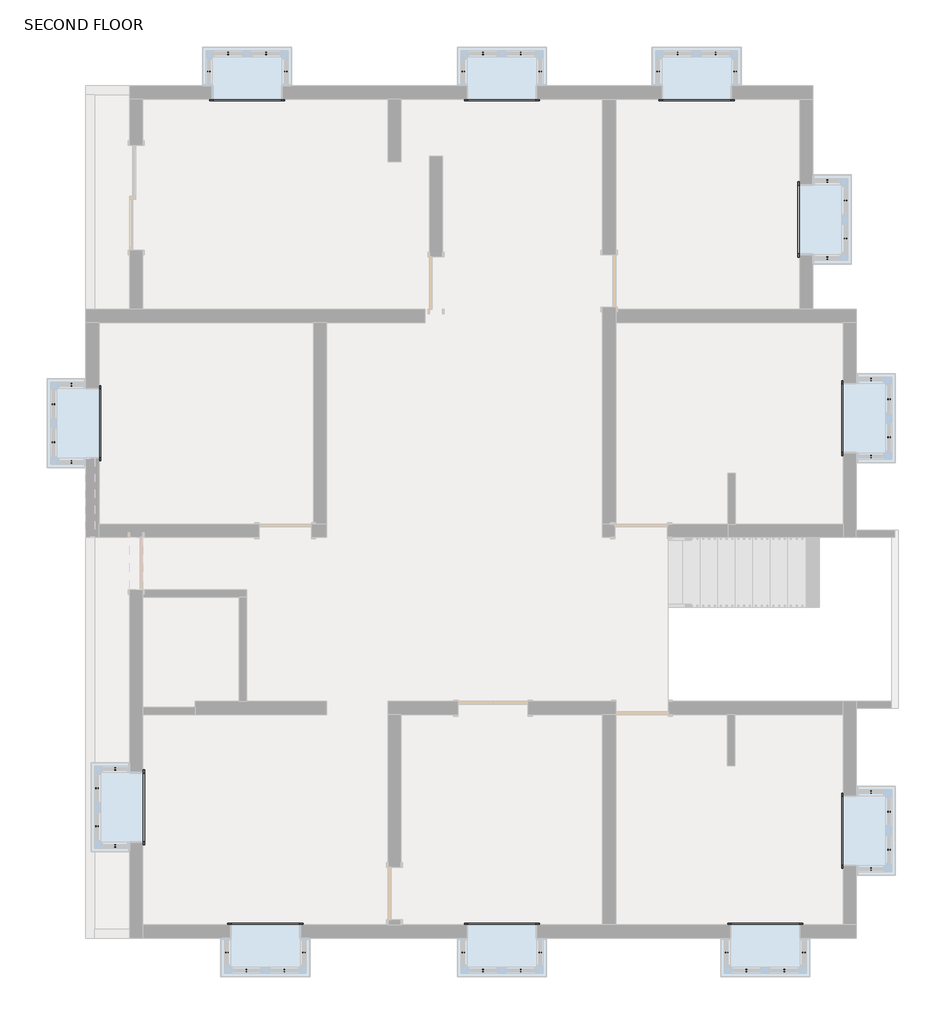
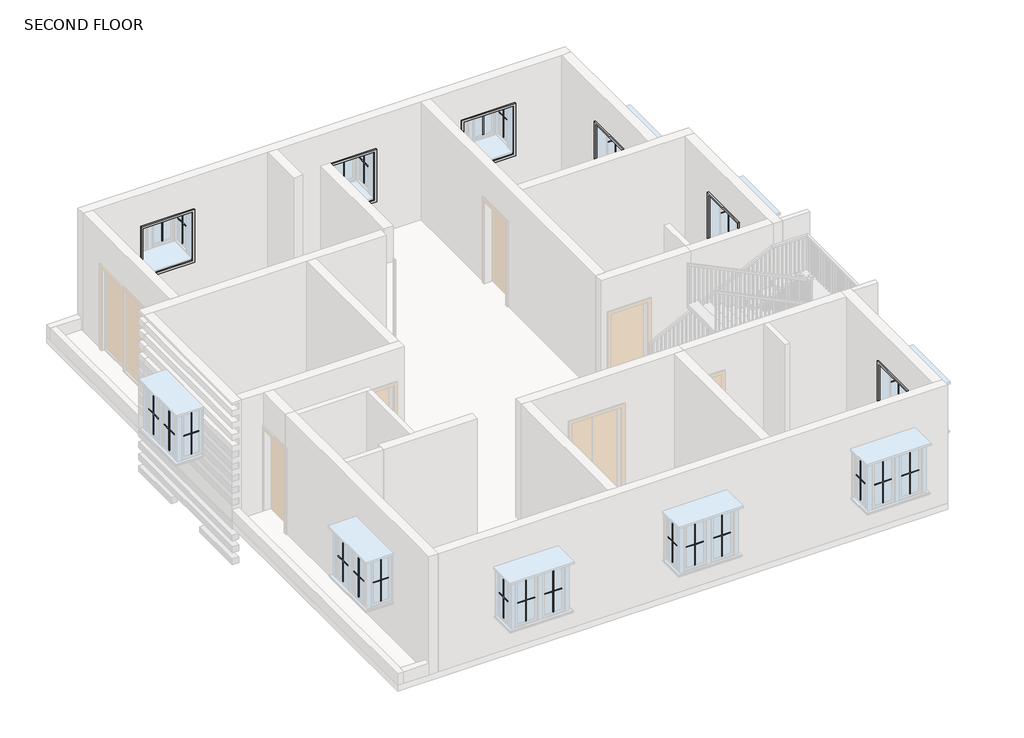
# One storey, part 6 of 6: 55 proxies.
"""IFC4 building model written with IfcOpenShell, lengths in millimetres."""

from ifc_helpers import new_model, si_unit, origin, place, context, project, spatial, transform, mapped, element, save
from components import muntin_pattern_2x2_muntin_pattern_2x2_4aee108e, muntin_pattern_2x2_muntin_pattern_2x2_f03ab90d, muntin_pattern_2x2_muntin_pattern_2x2_eb08c668, trim_window_interior_flat_picture_frame_ace0ae79

model = new_model("IFC4")

# Units and contexts
model_context = context("Model", 3, world=origin())
ifc_project = project(units=[si_unit("LENGTHUNIT", "METRE", prefix="MILLI")], contexts=[model_context])

# Site, building, storey
site = spatial("IfcSite", under=ifc_project)
building = spatial("IfcBuilding", under=site)
storey = spatial("IfcBuildingStorey", under=building, Name="SECOND FLOOR", Elevation=6400.8)

# Proxies
placement = place(None, origin())
muntin_pattern_2x2_muntin_pattern_2x2_shape = muntin_pattern_2x2_muntin_pattern_2x2_4aee108e(model_context)
element("IfcBuildingElementProxy", 1, Name="Muntin Pattern_2x2 : Muntin Pattern_2x2", ObjectType="Muntin Pattern_2x2 : Muntin Pattern_2x2", at=placement, inside=storey, context=model_context, shape_type="MappedRepresentation", body=[
    mapped(muntin_pattern_2x2_muntin_pattern_2x2_shape, transform((6209.1834916, 6075.433346, 7435.85), x_axis=(0.0, -1.0, 0.0), y_axis=(1.0, 0.0, 0.0), z_axis=(0.0, 0.0, 1.0))),
])
element("IfcBuildingElementProxy", 2, Name="Muntin Pattern_2x2 : Muntin Pattern_2x2", ObjectType="Muntin Pattern_2x2 : Muntin Pattern_2x2", at=placement, inside=storey, context=model_context, shape_type="MappedRepresentation", body=[
    mapped(muntin_pattern_2x2_muntin_pattern_2x2_shape, transform((-99.5415084, 8637.658346, 7435.85), x_axis=(1.0, 0.0, 0.0), y_axis=(0.0, 1.0, 0.0), z_axis=(0.0, 0.0, 1.0))),
])
element("IfcBuildingElementProxy", 3, Name="Muntin Pattern_2x2 : Muntin Pattern_2x2", ObjectType="Muntin Pattern_2x2 : Muntin Pattern_2x2", at=placement, inside=storey, context=model_context, shape_type="MappedRepresentation", body=[
    mapped(muntin_pattern_2x2_muntin_pattern_2x2_shape, transform((3291.3584916, 8637.658346, 7435.85), x_axis=(1.0, 0.0, 0.0), y_axis=(0.0, 1.0, 0.0), z_axis=(0.0, 0.0, 1.0))),
])
element("IfcBuildingElementProxy", 4, Name="Muntin Pattern_2x2 : Muntin Pattern_2x2", ObjectType="Muntin Pattern_2x2 : Muntin Pattern_2x2", at=placement, inside=storey, context=model_context, shape_type="MappedRepresentation", body=[
    mapped(muntin_pattern_2x2_muntin_pattern_2x2_shape, transform((-4531.8415084, 8637.658346, 7435.85), x_axis=(1.0, 0.0, 0.0), y_axis=(0.0, 1.0, 0.0), z_axis=(0.0, 0.0, 1.0))),
])
element("IfcBuildingElementProxy", 5, Name="Muntin Pattern_2x2 : Muntin Pattern_2x2", ObjectType="Muntin Pattern_2x2 : Muntin Pattern_2x2", at=placement, inside=storey, context=model_context, shape_type="MappedRepresentation", body=[
    mapped(muntin_pattern_2x2_muntin_pattern_2x2_shape, transform((-7576.6665084, 1871.733346, 7435.85), x_axis=(0.0, 1.0, 0.0), y_axis=(-1.0, 0.0, 0.0), z_axis=(0.0, 0.0, 1.0))),
])
element("IfcBuildingElementProxy", 6, Name="Muntin Pattern_2x2 : Muntin Pattern_2x2", ObjectType="Muntin Pattern_2x2 : Muntin Pattern_2x2", at=placement, inside=storey, context=model_context, shape_type="MappedRepresentation", body=[
    mapped(muntin_pattern_2x2_muntin_pattern_2x2_shape, transform((6971.1834916, 2621.033346, 7435.85), x_axis=(0.0, -1.0, 0.0), y_axis=(1.0, 0.0, 0.0), z_axis=(0.0, 0.0, 1.0))),
])
element("IfcBuildingElementProxy", 7, Name="Muntin Pattern_2x2 : Muntin Pattern_2x2", ObjectType="Muntin Pattern_2x2 : Muntin Pattern_2x2", at=placement, inside=storey, context=model_context, shape_type="MappedRepresentation", body=[
    mapped(muntin_pattern_2x2_muntin_pattern_2x2_shape, transform((-3553.9415084, -7319.891654, 7435.85), x_axis=(-1.0, 0.0, 0.0), y_axis=(0.0, -1.0, 0.0), z_axis=(0.0, 0.0, 1.0))),
])
element("IfcBuildingElementProxy", 8, Name="Muntin Pattern_2x2 : Muntin Pattern_2x2", ObjectType="Muntin Pattern_2x2 : Muntin Pattern_2x2", at=placement, inside=storey, context=model_context, shape_type="MappedRepresentation", body=[
    mapped(muntin_pattern_2x2_muntin_pattern_2x2_shape, transform((5145.5584916, -7319.891654, 7435.85), x_axis=(-1.0, 0.0, 0.0), y_axis=(0.0, -1.0, 0.0), z_axis=(0.0, 0.0, 1.0))),
])
element("IfcBuildingElementProxy", 9, Name="Muntin Pattern_2x2 : Muntin Pattern_2x2", ObjectType="Muntin Pattern_2x2 : Muntin Pattern_2x2", at=placement, inside=storey, context=model_context, shape_type="MappedRepresentation", body=[
    mapped(muntin_pattern_2x2_muntin_pattern_2x2_shape, transform((560.8584916, -7319.891654, 7435.85), x_axis=(-1.0, 0.0, 0.0), y_axis=(0.0, -1.0, 0.0), z_axis=(0.0, 0.0, 1.0))),
])
element("IfcBuildingElementProxy", 10, Name="Muntin Pattern_2x2 : Muntin Pattern_2x2", ObjectType="Muntin Pattern_2x2 : Muntin Pattern_2x2", at=placement, inside=storey, context=model_context, shape_type="MappedRepresentation", body=[
    mapped(muntin_pattern_2x2_muntin_pattern_2x2_shape, transform((-6814.6665084, -4808.466654, 7435.85), x_axis=(0.0, 1.0, 0.0), y_axis=(-1.0, 0.0, 0.0), z_axis=(0.0, 0.0, 1.0))),
])
element("IfcBuildingElementProxy", 11, Name="Muntin Pattern_2x2 : Muntin Pattern_2x2", ObjectType="Muntin Pattern_2x2 : Muntin Pattern_2x2", at=placement, inside=storey, context=model_context, shape_type="MappedRepresentation", body=[
    mapped(muntin_pattern_2x2_muntin_pattern_2x2_shape, transform((6971.1834916, -4554.466654, 7435.85), x_axis=(0.0, -1.0, 0.0), y_axis=(1.0, 0.0, 0.0), z_axis=(0.0, 0.0, 1.0))),
])
muntin_pattern_2x2_muntin_pattern_2x2_2_shape = muntin_pattern_2x2_muntin_pattern_2x2_f03ab90d(model_context)
element("IfcBuildingElementProxy", 12, Name="Muntin Pattern_2x2 : Muntin Pattern_2x2", ObjectType="Muntin Pattern_2x2 : Muntin Pattern_2x2", at=placement, inside=storey, context=model_context, shape_type="MappedRepresentation", body=[
    mapped(muntin_pattern_2x2_muntin_pattern_2x2_2_shape, transform((5894.8584916, 6415.158346, 7435.85), x_axis=(-1.0, 0.0, 0.0), y_axis=(0.0, -1.0, 0.0), z_axis=(0.0, 0.0, 1.0))),
])
element("IfcBuildingElementProxy", 13, Name="Muntin Pattern_2x2 : Muntin Pattern_2x2", ObjectType="Muntin Pattern_2x2 : Muntin Pattern_2x2", at=placement, inside=storey, context=model_context, shape_type="MappedRepresentation", body=[
    mapped(muntin_pattern_2x2_muntin_pattern_2x2_2_shape, transform((5894.8584916, 5075.308346, 7435.85), x_axis=(1.0, 0.0, 0.0), y_axis=(0.0, 1.0, 0.0), z_axis=(0.0, 0.0, 1.0))),
])
element("IfcBuildingElementProxy", 14, Name="Muntin Pattern_2x2 : Muntin Pattern_2x2", ObjectType="Muntin Pattern_2x2 : Muntin Pattern_2x2", at=placement, inside=storey, context=model_context, shape_type="MappedRepresentation", body=[
    mapped(muntin_pattern_2x2_muntin_pattern_2x2_2_shape, transform((-439.2665084, 8323.333346, 7435.85), x_axis=(0.0, -1.0, 0.0), y_axis=(1.0, 0.0, 0.0), z_axis=(0.0, 0.0, 1.0))),
])
element("IfcBuildingElementProxy", 15, Name="Muntin Pattern_2x2 : Muntin Pattern_2x2", ObjectType="Muntin Pattern_2x2 : Muntin Pattern_2x2", at=placement, inside=storey, context=model_context, shape_type="MappedRepresentation", body=[
    mapped(muntin_pattern_2x2_muntin_pattern_2x2_2_shape, transform((900.5834916, 8323.333346, 7435.85), x_axis=(0.0, 1.0, 0.0), y_axis=(-1.0, 0.0, 0.0), z_axis=(0.0, 0.0, 1.0))),
])
element("IfcBuildingElementProxy", 16, Name="Muntin Pattern_2x2 : Muntin Pattern_2x2", ObjectType="Muntin Pattern_2x2 : Muntin Pattern_2x2", at=placement, inside=storey, context=model_context, shape_type="MappedRepresentation", body=[
    mapped(muntin_pattern_2x2_muntin_pattern_2x2_2_shape, transform((2951.6334916, 8323.333346, 7435.85), x_axis=(0.0, -1.0, 0.0), y_axis=(1.0, 0.0, 0.0), z_axis=(0.0, 0.0, 1.0))),
])
element("IfcBuildingElementProxy", 17, Name="Muntin Pattern_2x2 : Muntin Pattern_2x2", ObjectType="Muntin Pattern_2x2 : Muntin Pattern_2x2", at=placement, inside=storey, context=model_context, shape_type="MappedRepresentation", body=[
    mapped(muntin_pattern_2x2_muntin_pattern_2x2_2_shape, transform((4291.4834916, 8323.333346, 7435.85), x_axis=(0.0, 1.0, 0.0), y_axis=(-1.0, 0.0, 0.0), z_axis=(0.0, 0.0, 1.0))),
])
element("IfcBuildingElementProxy", 18, Name="Muntin Pattern_2x2 : Muntin Pattern_2x2", ObjectType="Muntin Pattern_2x2 : Muntin Pattern_2x2", at=placement, inside=storey, context=model_context, shape_type="MappedRepresentation", body=[
    mapped(muntin_pattern_2x2_muntin_pattern_2x2_2_shape, transform((-4871.5665084, 8323.333346, 7435.85), x_axis=(0.0, -1.0, 0.0), y_axis=(1.0, 0.0, 0.0), z_axis=(0.0, 0.0, 1.0))),
])
element("IfcBuildingElementProxy", 19, Name="Muntin Pattern_2x2 : Muntin Pattern_2x2", ObjectType="Muntin Pattern_2x2 : Muntin Pattern_2x2", at=placement, inside=storey, context=model_context, shape_type="MappedRepresentation", body=[
    mapped(muntin_pattern_2x2_muntin_pattern_2x2_2_shape, transform((-3531.7165084, 8323.333346, 7435.85), x_axis=(0.0, 1.0, 0.0), y_axis=(-1.0, 0.0, 0.0), z_axis=(0.0, 0.0, 1.0))),
])
element("IfcBuildingElementProxy", 20, Name="Muntin Pattern_2x2 : Muntin Pattern_2x2", ObjectType="Muntin Pattern_2x2 : Muntin Pattern_2x2", at=placement, inside=storey, context=model_context, shape_type="MappedRepresentation", body=[
    mapped(muntin_pattern_2x2_muntin_pattern_2x2_2_shape, transform((-7262.3415084, 1532.008346, 7435.85), x_axis=(1.0, 0.0, 0.0), y_axis=(0.0, 1.0, 0.0), z_axis=(0.0, 0.0, 1.0))),
])
element("IfcBuildingElementProxy", 21, Name="Muntin Pattern_2x2 : Muntin Pattern_2x2", ObjectType="Muntin Pattern_2x2 : Muntin Pattern_2x2", at=placement, inside=storey, context=model_context, shape_type="MappedRepresentation", body=[
    mapped(muntin_pattern_2x2_muntin_pattern_2x2_2_shape, transform((-7262.3415084, 2871.858346, 7435.85), x_axis=(-1.0, 0.0, 0.0), y_axis=(0.0, -1.0, 0.0), z_axis=(0.0, 0.0, 1.0))),
])
element("IfcBuildingElementProxy", 22, Name="Muntin Pattern_2x2 : Muntin Pattern_2x2", ObjectType="Muntin Pattern_2x2 : Muntin Pattern_2x2", at=placement, inside=storey, context=model_context, shape_type="MappedRepresentation", body=[
    mapped(muntin_pattern_2x2_muntin_pattern_2x2_2_shape, transform((6656.8584916, 2960.758346, 7435.85), x_axis=(-1.0, 0.0, 0.0), y_axis=(0.0, -1.0, 0.0), z_axis=(0.0, 0.0, 1.0))),
])
element("IfcBuildingElementProxy", 23, Name="Muntin Pattern_2x2 : Muntin Pattern_2x2", ObjectType="Muntin Pattern_2x2 : Muntin Pattern_2x2", at=placement, inside=storey, context=model_context, shape_type="MappedRepresentation", body=[
    mapped(muntin_pattern_2x2_muntin_pattern_2x2_2_shape, transform((6656.8584916, 1620.908346, 7435.85), x_axis=(1.0, 0.0, 0.0), y_axis=(0.0, 1.0, 0.0), z_axis=(0.0, 0.0, 1.0))),
])
element("IfcBuildingElementProxy", 24, Name="Muntin Pattern_2x2 : Muntin Pattern_2x2", ObjectType="Muntin Pattern_2x2 : Muntin Pattern_2x2", at=placement, inside=storey, context=model_context, shape_type="MappedRepresentation", body=[
    mapped(muntin_pattern_2x2_muntin_pattern_2x2_2_shape, transform((-3214.2165084, -7005.566654, 7435.85), x_axis=(0.0, 1.0, 0.0), y_axis=(-1.0, 0.0, 0.0), z_axis=(0.0, 0.0, 1.0))),
])
element("IfcBuildingElementProxy", 25, Name="Muntin Pattern_2x2 : Muntin Pattern_2x2", ObjectType="Muntin Pattern_2x2 : Muntin Pattern_2x2", at=placement, inside=storey, context=model_context, shape_type="MappedRepresentation", body=[
    mapped(muntin_pattern_2x2_muntin_pattern_2x2_2_shape, transform((-4554.0665084, -7005.566654, 7435.85), x_axis=(0.0, -1.0, 0.0), y_axis=(1.0, 0.0, 0.0), z_axis=(0.0, 0.0, 1.0))),
])
element("IfcBuildingElementProxy", 26, Name="Muntin Pattern_2x2 : Muntin Pattern_2x2", ObjectType="Muntin Pattern_2x2 : Muntin Pattern_2x2", at=placement, inside=storey, context=model_context, shape_type="MappedRepresentation", body=[
    mapped(muntin_pattern_2x2_muntin_pattern_2x2_2_shape, transform((5485.2834916, -7005.566654, 7435.85), x_axis=(0.0, 1.0, 0.0), y_axis=(-1.0, 0.0, 0.0), z_axis=(0.0, 0.0, 1.0))),
])
element("IfcBuildingElementProxy", 27, Name="Muntin Pattern_2x2 : Muntin Pattern_2x2", ObjectType="Muntin Pattern_2x2 : Muntin Pattern_2x2", at=placement, inside=storey, context=model_context, shape_type="MappedRepresentation", body=[
    mapped(muntin_pattern_2x2_muntin_pattern_2x2_2_shape, transform((4145.4334916, -7005.566654, 7435.85), x_axis=(0.0, -1.0, 0.0), y_axis=(1.0, 0.0, 0.0), z_axis=(0.0, 0.0, 1.0))),
])
element("IfcBuildingElementProxy", 28, Name="Muntin Pattern_2x2 : Muntin Pattern_2x2", ObjectType="Muntin Pattern_2x2 : Muntin Pattern_2x2", at=placement, inside=storey, context=model_context, shape_type="MappedRepresentation", body=[
    mapped(muntin_pattern_2x2_muntin_pattern_2x2_2_shape, transform((900.5834916, -7005.566654, 7435.85), x_axis=(0.0, 1.0, 0.0), y_axis=(-1.0, 0.0, 0.0), z_axis=(0.0, 0.0, 1.0))),
])
element("IfcBuildingElementProxy", 29, Name="Muntin Pattern_2x2 : Muntin Pattern_2x2", ObjectType="Muntin Pattern_2x2 : Muntin Pattern_2x2", at=placement, inside=storey, context=model_context, shape_type="MappedRepresentation", body=[
    mapped(muntin_pattern_2x2_muntin_pattern_2x2_2_shape, transform((-439.2665084, -7005.566654, 7435.85), x_axis=(0.0, -1.0, 0.0), y_axis=(1.0, 0.0, 0.0), z_axis=(0.0, 0.0, 1.0))),
])
element("IfcBuildingElementProxy", 30, Name="Muntin Pattern_2x2 : Muntin Pattern_2x2", ObjectType="Muntin Pattern_2x2 : Muntin Pattern_2x2", at=placement, inside=storey, context=model_context, shape_type="MappedRepresentation", body=[
    mapped(muntin_pattern_2x2_muntin_pattern_2x2_2_shape, transform((-6500.3415084, -5148.191654, 7435.85), x_axis=(1.0, 0.0, 0.0), y_axis=(0.0, 1.0, 0.0), z_axis=(0.0, 0.0, 1.0))),
])
element("IfcBuildingElementProxy", 31, Name="Muntin Pattern_2x2 : Muntin Pattern_2x2", ObjectType="Muntin Pattern_2x2 : Muntin Pattern_2x2", at=placement, inside=storey, context=model_context, shape_type="MappedRepresentation", body=[
    mapped(muntin_pattern_2x2_muntin_pattern_2x2_2_shape, transform((-6500.3415084, -3808.341654, 7435.85), x_axis=(-1.0, 0.0, 0.0), y_axis=(0.0, -1.0, 0.0), z_axis=(0.0, 0.0, 1.0))),
])
element("IfcBuildingElementProxy", 32, Name="Muntin Pattern_2x2 : Muntin Pattern_2x2", ObjectType="Muntin Pattern_2x2 : Muntin Pattern_2x2", at=placement, inside=storey, context=model_context, shape_type="MappedRepresentation", body=[
    mapped(muntin_pattern_2x2_muntin_pattern_2x2_2_shape, transform((6656.8584916, -4214.741654, 7435.85), x_axis=(-1.0, 0.0, 0.0), y_axis=(0.0, -1.0, 0.0), z_axis=(0.0, 0.0, 1.0))),
])
element("IfcBuildingElementProxy", 33, Name="Muntin Pattern_2x2 : Muntin Pattern_2x2", ObjectType="Muntin Pattern_2x2 : Muntin Pattern_2x2", at=placement, inside=storey, context=model_context, shape_type="MappedRepresentation", body=[
    mapped(muntin_pattern_2x2_muntin_pattern_2x2_2_shape, transform((6656.8584916, -5554.591654, 7435.85), x_axis=(1.0, 0.0, 0.0), y_axis=(0.0, 1.0, 0.0), z_axis=(0.0, 0.0, 1.0))),
])
muntin_pattern_2x2_muntin_pattern_2x2_3_shape = muntin_pattern_2x2_muntin_pattern_2x2_eb08c668(model_context)
element("IfcBuildingElementProxy", 34, Name="Muntin Pattern_2x2 : Muntin Pattern_2x2", ObjectType="Muntin Pattern_2x2 : Muntin Pattern_2x2", at=placement, inside=storey, context=model_context, shape_type="MappedRepresentation", body=[
    mapped(muntin_pattern_2x2_muntin_pattern_2x2_3_shape, transform((6209.1834916, 5415.033346, 7435.85), x_axis=(0.0, 1.0, 0.0), y_axis=(-1.0, 0.0, 0.0), z_axis=(0.0, 0.0, 1.0))),
])
element("IfcBuildingElementProxy", 35, Name="Muntin Pattern_2x2 : Muntin Pattern_2x2", ObjectType="Muntin Pattern_2x2 : Muntin Pattern_2x2", at=placement, inside=storey, context=model_context, shape_type="MappedRepresentation", body=[
    mapped(muntin_pattern_2x2_muntin_pattern_2x2_3_shape, transform((560.8584916, 8637.658346, 7435.85), x_axis=(-1.0, 0.0, 0.0), y_axis=(0.0, -1.0, 0.0), z_axis=(0.0, 0.0, 1.0))),
])
element("IfcBuildingElementProxy", 36, Name="Muntin Pattern_2x2 : Muntin Pattern_2x2", ObjectType="Muntin Pattern_2x2 : Muntin Pattern_2x2", at=placement, inside=storey, context=model_context, shape_type="MappedRepresentation", body=[
    mapped(muntin_pattern_2x2_muntin_pattern_2x2_3_shape, transform((3951.7584916, 8637.658346, 7435.85), x_axis=(-1.0, 0.0, 0.0), y_axis=(0.0, -1.0, 0.0), z_axis=(0.0, 0.0, 1.0))),
])
element("IfcBuildingElementProxy", 37, Name="Muntin Pattern_2x2 : Muntin Pattern_2x2", ObjectType="Muntin Pattern_2x2 : Muntin Pattern_2x2", at=placement, inside=storey, context=model_context, shape_type="MappedRepresentation", body=[
    mapped(muntin_pattern_2x2_muntin_pattern_2x2_3_shape, transform((-3871.4415084, 8637.658346, 7435.85), x_axis=(-1.0, 0.0, 0.0), y_axis=(0.0, -1.0, 0.0), z_axis=(0.0, 0.0, 1.0))),
])
element("IfcBuildingElementProxy", 38, Name="Muntin Pattern_2x2 : Muntin Pattern_2x2", ObjectType="Muntin Pattern_2x2 : Muntin Pattern_2x2", at=placement, inside=storey, context=model_context, shape_type="MappedRepresentation", body=[
    mapped(muntin_pattern_2x2_muntin_pattern_2x2_3_shape, transform((-7576.6665084, 2532.133346, 7435.85), x_axis=(0.0, -1.0, 0.0), y_axis=(1.0, 0.0, 0.0), z_axis=(0.0, 0.0, 1.0))),
])
element("IfcBuildingElementProxy", 39, Name="Muntin Pattern_2x2 : Muntin Pattern_2x2", ObjectType="Muntin Pattern_2x2 : Muntin Pattern_2x2", at=placement, inside=storey, context=model_context, shape_type="MappedRepresentation", body=[
    mapped(muntin_pattern_2x2_muntin_pattern_2x2_3_shape, transform((6971.1834916, 1960.633346, 7435.85), x_axis=(0.0, 1.0, 0.0), y_axis=(-1.0, 0.0, 0.0), z_axis=(0.0, 0.0, 1.0))),
])
element("IfcBuildingElementProxy", 40, Name="Muntin Pattern_2x2 : Muntin Pattern_2x2", ObjectType="Muntin Pattern_2x2 : Muntin Pattern_2x2", at=placement, inside=storey, context=model_context, shape_type="MappedRepresentation", body=[
    mapped(muntin_pattern_2x2_muntin_pattern_2x2_3_shape, transform((-4214.3415084, -7319.891654, 7435.85), x_axis=(1.0, 0.0, 0.0), y_axis=(0.0, 1.0, 0.0), z_axis=(0.0, 0.0, 1.0))),
])
element("IfcBuildingElementProxy", 41, Name="Muntin Pattern_2x2 : Muntin Pattern_2x2", ObjectType="Muntin Pattern_2x2 : Muntin Pattern_2x2", at=placement, inside=storey, context=model_context, shape_type="MappedRepresentation", body=[
    mapped(muntin_pattern_2x2_muntin_pattern_2x2_3_shape, transform((4485.1584916, -7319.891654, 7435.85), x_axis=(1.0, 0.0, 0.0), y_axis=(0.0, 1.0, 0.0), z_axis=(0.0, 0.0, 1.0))),
])
element("IfcBuildingElementProxy", 42, Name="Muntin Pattern_2x2 : Muntin Pattern_2x2", ObjectType="Muntin Pattern_2x2 : Muntin Pattern_2x2", at=placement, inside=storey, context=model_context, shape_type="MappedRepresentation", body=[
    mapped(muntin_pattern_2x2_muntin_pattern_2x2_3_shape, transform((-99.5415084, -7319.891654, 7435.85), x_axis=(1.0, 0.0, 0.0), y_axis=(0.0, 1.0, 0.0), z_axis=(0.0, 0.0, 1.0))),
])
element("IfcBuildingElementProxy", 43, Name="Muntin Pattern_2x2 : Muntin Pattern_2x2", ObjectType="Muntin Pattern_2x2 : Muntin Pattern_2x2", at=placement, inside=storey, context=model_context, shape_type="MappedRepresentation", body=[
    mapped(muntin_pattern_2x2_muntin_pattern_2x2_3_shape, transform((-6814.6665084, -4148.066654, 7435.85), x_axis=(0.0, -1.0, 0.0), y_axis=(1.0, 0.0, 0.0), z_axis=(0.0, 0.0, 1.0))),
])
element("IfcBuildingElementProxy", 44, Name="Muntin Pattern_2x2 : Muntin Pattern_2x2", ObjectType="Muntin Pattern_2x2 : Muntin Pattern_2x2", at=placement, inside=storey, context=model_context, shape_type="MappedRepresentation", body=[
    mapped(muntin_pattern_2x2_muntin_pattern_2x2_3_shape, transform((6971.1834916, -5214.866654, 7435.85), x_axis=(0.0, 1.0, 0.0), y_axis=(-1.0, 0.0, 0.0), z_axis=(0.0, 0.0, 1.0))),
])
trim_window_interior_flat_picture_frame_shape = trim_window_interior_flat_picture_frame_ace0ae79(model_context)
element("IfcBuildingElementProxy", 45, Name="Trim-Window-Interior-Flat : Picture Frame", ObjectType="Trim-Window-Interior-Flat : Picture Frame", at=placement, inside=storey, context=model_context, shape_type="MappedRepresentation", body=[
    mapped(trim_window_interior_flat_picture_frame_shape, transform((5412.2584916, 5745.233346, 8585.2), x_axis=(0.0, -1.0, 0.0), y_axis=(0.0, 0.0, 1.0), z_axis=(-1.0, 0.0, 0.0))),
])
element("IfcBuildingElementProxy", 46, Name="Trim-Window-Interior-Flat : Picture Frame", ObjectType="Trim-Window-Interior-Flat : Picture Frame", at=placement, inside=storey, context=model_context, shape_type="MappedRepresentation", body=[
    mapped(trim_window_interior_flat_picture_frame_shape, transform((230.6584916, 7840.733346, 8585.2), x_axis=(1.0, 0.0, 0.0), y_axis=(0.0, 0.0, 1.0), z_axis=(0.0, -1.0, 0.0))),
])
element("IfcBuildingElementProxy", 47, Name="Trim-Window-Interior-Flat : Picture Frame", ObjectType="Trim-Window-Interior-Flat : Picture Frame", at=placement, inside=storey, context=model_context, shape_type="MappedRepresentation", body=[
    mapped(trim_window_interior_flat_picture_frame_shape, transform((3621.5584916, 7840.733346, 8585.2), x_axis=(1.0, 0.0, 0.0), y_axis=(0.0, 0.0, 1.0), z_axis=(0.0, -1.0, 0.0))),
])
element("IfcBuildingElementProxy", 48, Name="Trim-Window-Interior-Flat : Picture Frame", ObjectType="Trim-Window-Interior-Flat : Picture Frame", at=placement, inside=storey, context=model_context, shape_type="MappedRepresentation", body=[
    mapped(trim_window_interior_flat_picture_frame_shape, transform((-4201.6415084, 7840.733346, 8585.2), x_axis=(1.0, 0.0, 0.0), y_axis=(0.0, 0.0, 1.0), z_axis=(0.0, -1.0, 0.0))),
])
element("IfcBuildingElementProxy", 49, Name="Trim-Window-Interior-Flat : Picture Frame", ObjectType="Trim-Window-Interior-Flat : Picture Frame", at=placement, inside=storey, context=model_context, shape_type="MappedRepresentation", body=[
    mapped(trim_window_interior_flat_picture_frame_shape, transform((-6779.7415084, 2201.933346, 8585.2), x_axis=(0.0, 1.0, 0.0), y_axis=(0.0, 0.0, 1.0), z_axis=(1.0, 0.0, 0.0))),
])
element("IfcBuildingElementProxy", 50, Name="Trim-Window-Interior-Flat : Picture Frame", ObjectType="Trim-Window-Interior-Flat : Picture Frame", at=placement, inside=storey, context=model_context, shape_type="MappedRepresentation", body=[
    mapped(trim_window_interior_flat_picture_frame_shape, transform((6174.2584916, 2290.833346, 8585.2), x_axis=(0.0, -1.0, 0.0), y_axis=(0.0, 0.0, 1.0), z_axis=(-1.0, 0.0, 0.0))),
])
element("IfcBuildingElementProxy", 51, Name="Trim-Window-Interior-Flat : Picture Frame", ObjectType="Trim-Window-Interior-Flat : Picture Frame", at=placement, inside=storey, context=model_context, shape_type="MappedRepresentation", body=[
    mapped(trim_window_interior_flat_picture_frame_shape, transform((-3884.1415084, -6522.966654, 8585.2), x_axis=(-1.0, 0.0, 0.0), y_axis=(0.0, 0.0, 1.0), z_axis=(0.0, 1.0, 0.0))),
])
element("IfcBuildingElementProxy", 52, Name="Trim-Window-Interior-Flat : Picture Frame", ObjectType="Trim-Window-Interior-Flat : Picture Frame", at=placement, inside=storey, context=model_context, shape_type="MappedRepresentation", body=[
    mapped(trim_window_interior_flat_picture_frame_shape, transform((4815.3584916, -6522.966654, 8585.2), x_axis=(-1.0, 0.0, 0.0), y_axis=(0.0, 0.0, 1.0), z_axis=(0.0, 1.0, 0.0))),
])
element("IfcBuildingElementProxy", 53, Name="Trim-Window-Interior-Flat : Picture Frame", ObjectType="Trim-Window-Interior-Flat : Picture Frame", at=placement, inside=storey, context=model_context, shape_type="MappedRepresentation", body=[
    mapped(trim_window_interior_flat_picture_frame_shape, transform((230.6584916, -6522.966654, 8585.2), x_axis=(-1.0, 0.0, 0.0), y_axis=(0.0, 0.0, 1.0), z_axis=(0.0, 1.0, 0.0))),
])
element("IfcBuildingElementProxy", 54, Name="Trim-Window-Interior-Flat : Picture Frame", ObjectType="Trim-Window-Interior-Flat : Picture Frame", at=placement, inside=storey, context=model_context, shape_type="MappedRepresentation", body=[
    mapped(trim_window_interior_flat_picture_frame_shape, transform((-6017.7415084, -4478.266654, 8585.2), x_axis=(0.0, 1.0, 0.0), y_axis=(0.0, 0.0, 1.0), z_axis=(1.0, 0.0, 0.0))),
])
element("IfcBuildingElementProxy", 55, Name="Trim-Window-Interior-Flat : Picture Frame", ObjectType="Trim-Window-Interior-Flat : Picture Frame", at=placement, inside=storey, context=model_context, shape_type="MappedRepresentation", body=[
    mapped(trim_window_interior_flat_picture_frame_shape, transform((6174.2584916, -4884.666654, 8585.2), x_axis=(0.0, -1.0, 0.0), y_axis=(0.0, 0.0, 1.0), z_axis=(-1.0, 0.0, 0.0))),
])

save(model, "model.ifc")

# Revit data of these elements
# Type "Muntin Pattern_2x2 : Muntin Pattern_2x2"
#   Width [instance default] = 4' - 0"
#   Thickness = 0' - 0 1/2"
#   Height [instance default] = 4' - 0"
#   Distance = 0' - 0 3/4"
#   Interior Material [instance default] = none
#   Exterior Material [instance default] = none
#   Default Elevation = 0
# Type "Trim-Window-Interior-Flat : Picture Frame"
#   Trim Thickness_Picture Frame = 0' - 1 1/4"
#   Trim Width = 0' - 2 1/4"
#   Trim Thickness_with Sill = 0' - 0 3/4"
#   Sill Thickness = 0' - 1 1/4"
#   Opening Width [instance default] = 2' - 0"
#   Opening Height [instance default] = 3' - 0"
#   Default Elevation = 4' - 0"
#   Sill = no
#   Picture Frame = yes
#   Trim Material [instance default] = none
# Elements 1, 2, 3, 4, 5, 6, 7, 8, 9, 10, 11, 34, 35, 36, 37, 38, 39, 40, 41, 42, 43, 44 (IfcBuildingElementProxy, "Muntin Pattern_2x2 : Muntin Pattern_2x2")
#   Width = 1' - 4 1/2"
#   Height = 3' - 6 1/2"
#   Interior Material = Wood - Stained
#   Exterior Material = Clad - White
#   Phase Created = New Construction
#   Materials on its faces: "Clad - White", "Wood - Stained"
# Elements 12, 13, 14, 15, 16, 17, 18, 19, 20, 21, 22, 23, 24, 25, 26, 27, 28, 29, 30, 31, 32, 33 (IfcBuildingElementProxy, "Muntin Pattern_2x2 : Muntin Pattern_2x2")
#   Width = 1' - 2 1/2"
#   Height = 3' - 6 1/2"
#   Interior Material = Wood - Stained
#   Exterior Material = Clad - White
#   Phase Created = New Construction
#   Materials on its faces: "Clad - White", "Wood - Stained"
# Elements 45, 46, 47, 48, 49, 50, 51, 52, 53, 54, 55 (IfcBuildingElementProxy, "Trim-Window-Interior-Flat : Picture Frame")
#   Opening Width = 4' - 0"
#   Opening Height = 4' - 2"
#   Trim Material = Wood - Stained
#   Phase Created = New Construction
#   Materials on its faces: "Wood - Stained"
# Materials
#   "Clad - White": class "Wood", colour RGB 242 242 238, transparency 0, Cost = 0
#   "Wood - Stained": class "Wood", colour RGB 224 178 126, transparency 0, Cost = 0
